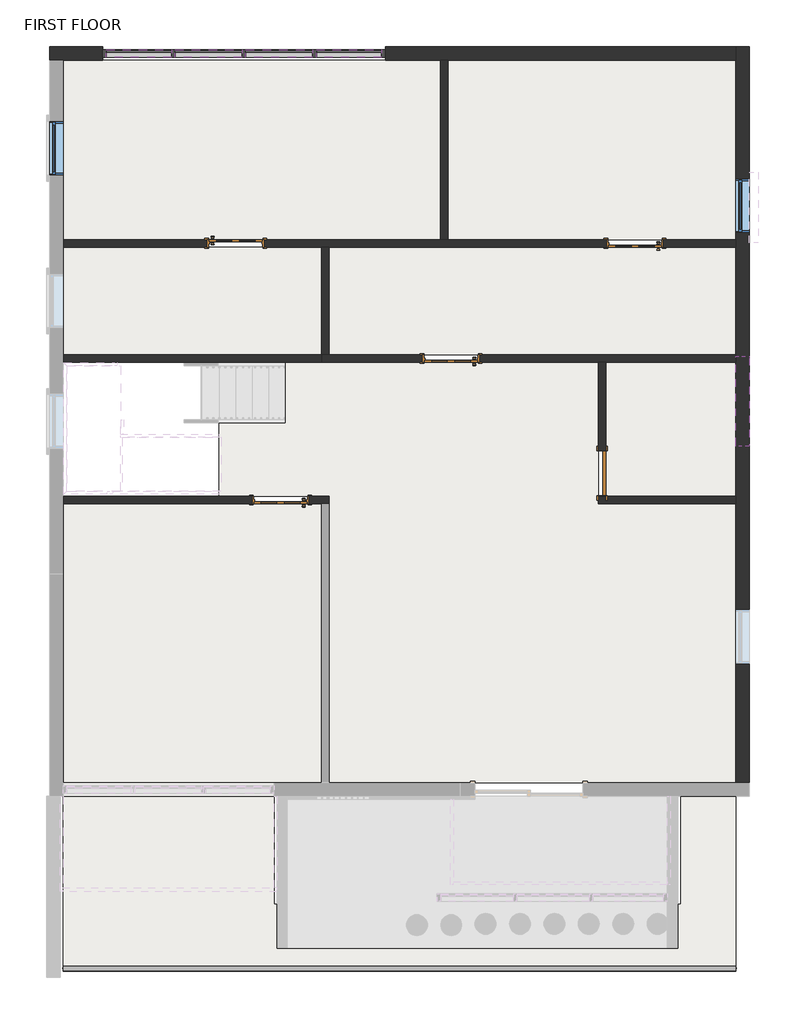
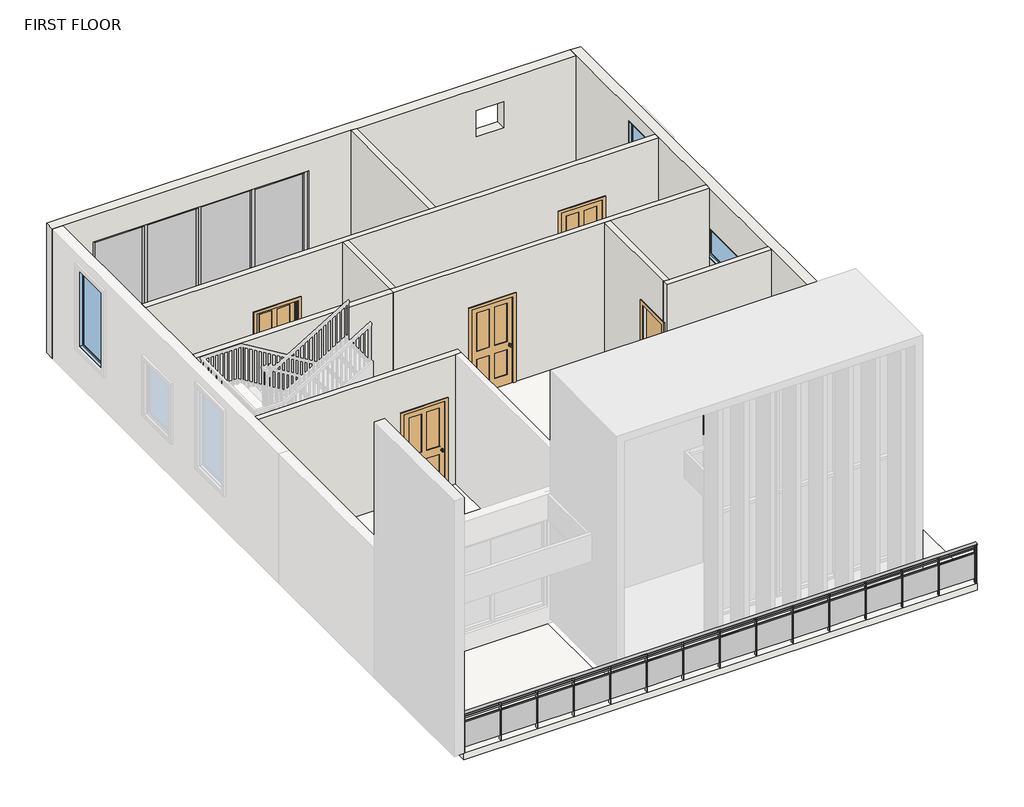
# One storey, part 2 of 4: 13 members, 10 walls, 5 doors, 4 plates, 3 windows, 1 railing, 1 slab.
"""IFC4 building model written with IfcOpenShell, lengths in millimetres."""

from ifc_helpers import new_model, si_unit, point, frame, origin, place, context, project, spatial, polyline, ellipse_curve, trimmed, outline, extrude, faceted_brep, transform, mapped, element, save
from ifc_brep_helpers import plane_surface, extruded_surface, advanced_brep
from components import door_65ef8926, door_1fe7f57d, member_d69c7880, member_a8685e1c, member_189d47d0, member_5afaafd3, system_panel_glazed_d43da186, system_panel_glazed_a1d10a75, window_2e8ca8a3, window_e88f44c6

model = new_model("IFC4")

# Units and contexts
model_context = context("Model", 3, world=origin())
ifc_project = project(units=[si_unit("LENGTHUNIT", "METRE", prefix="MILLI")], contexts=[model_context])

# Site, building, storey
site = spatial("IfcSite", under=ifc_project)
building = spatial("IfcBuilding", under=site)
storey = spatial("IfcBuildingStorey", under=building, Name="FIRST FLOOR", Elevation=3352.8)

# Doors
placement = place(None, origin())
door_shape = door_65ef8926(model_context)
element("IfcDoor", 1, ObjectType="Door-Interior-Single-4_Panel-Wood : 36\" x 80\"", at=placement, inside=storey, context=model_context, shape_type="MappedRepresentation", body=[
    mapped(door_shape, transform((-6068.2781265, 636.4415128, 3352.8), x_axis=(-1.0, 0.0, 0.0), y_axis=(0.0, -1.0, 0.0), z_axis=(0.0, 0.0, 1.0))),
])
element("IfcDoor", 2, ObjectType="Door-Interior-Single-4_Panel-Wood : 36\" x 80\"", at=placement, inside=storey, context=model_context, shape_type="MappedRepresentation", body=[
    mapped(door_shape, transform((-3172.6781265, 3037.1107468, 3352.8), x_axis=(-1.0, 0.0, 0.0), y_axis=(0.0, -1.0, 0.0), z_axis=(0.0, 0.0, 1.0))),
])
element("IfcDoor", 3, ObjectType="Door-Interior-Single-4_Panel-Wood : 36\" x 80\"", at=placement, inside=storey, context=model_context, shape_type="MappedRepresentation", body=[
    mapped(door_shape, transform((-6830.2781265, 4999.2607468, 3352.8), x_axis=(1.0, 0.0, 0.0), y_axis=(0.0, 1.0, 0.0), z_axis=(0.0, 0.0, 1.0))),
])
element("IfcDoor", 4, ObjectType="Door-Interior-Single-4_Panel-Wood : 36\" x 80\"", at=placement, inside=storey, context=model_context, shape_type="MappedRepresentation", body=[
    mapped(door_shape, transform((-48.4781265, 4992.9107468, 3352.8), x_axis=(-1.0, 0.0, 0.0), y_axis=(0.0, -1.0, 0.0), z_axis=(0.0, 0.0, 1.0))),
])
door_2_shape = door_1fe7f57d(model_context)
element("IfcDoor", 5, ObjectType="Single-Flush : 30\" x 80\"", at=placement, inside=storey, context=model_context, shape_type="MappedRepresentation", body=[
    mapped(door_2_shape, transform((-607.2781265, 1096.8165128, 3352.8), x_axis=(0.0, -1.0, 0.0), y_axis=(1.0, 0.0, 0.0), z_axis=(0.0, 0.0, 1.0))),
])

# Members
member_shape = member_d69c7880(model_context)
element("IfcMember", 6, ObjectType="Rectangular Mullion : 2.5\" x 5\" rectangular", at=placement, inside=storey, context=model_context, shape_type="MappedRepresentation", body=[
    mapped(member_shape, transform((-4353.7781265, 8221.8857468, 5781.7640157), x_axis=(0.0, 0.0, 1.0), y_axis=(0.0, -1.0, 0.0), z_axis=(1.0, 0.0, 0.0))),
])
element("IfcMember", 7, ObjectType="Rectangular Mullion : 2.5\" x 5\" rectangular", at=placement, inside=storey, context=model_context, shape_type="MappedRepresentation", body=[
    mapped(member_shape, transform((-7922.4781263, 8221.8857468, 5781.7640157), x_axis=(0.0, 0.0, 1.0), y_axis=(0.0, -1.0, 0.0), z_axis=(1.0, 0.0, 0.0))),
])
member_2_shape = member_a8685e1c(model_context)
element("IfcMember", 8, ObjectType="Rectangular Mullion : 2.5\" x 5\" rectangular", at=placement, inside=storey, context=model_context, shape_type="MappedRepresentation", body=[
    mapped(member_2_shape, transform((-6722.3281265, 8221.8857468, 5781.7640157), x_axis=(0.0, 0.0, 1.0), y_axis=(0.0, -1.0, 0.0), z_axis=(1.0, 0.0, 0.0))),
])
element("IfcMember", 9, ObjectType="Rectangular Mullion : 2.5\" x 5\" rectangular", at=placement, inside=storey, context=model_context, shape_type="MappedRepresentation", body=[
    mapped(member_2_shape, transform((-5522.1781266, 8221.8857468, 5781.7640157), x_axis=(0.0, 0.0, 1.0), y_axis=(0.0, -1.0, 0.0), z_axis=(1.0, 0.0, 0.0))),
])
element("IfcMember", 10, ObjectType="Rectangular Mullion : 2.5\" x 5\" rectangular", at=placement, inside=storey, context=model_context, shape_type="MappedRepresentation", body=[
    mapped(member_shape, transform((-9027.3781265, 8221.8857468, 3352.8), x_axis=(0.0, 0.0, -1.0), y_axis=(0.0, -1.0, 0.0), z_axis=(-1.0, 0.0, 0.0))),
])
element("IfcMember", 11, ObjectType="Rectangular Mullion : 2.5\" x 5\" rectangular", at=placement, inside=storey, context=model_context, shape_type="MappedRepresentation", body=[
    mapped(member_shape, transform((-5458.6781266, 8221.8857468, 3352.8), x_axis=(0.0, 0.0, -1.0), y_axis=(0.0, -1.0, 0.0), z_axis=(-1.0, 0.0, 0.0))),
])
element("IfcMember", 12, ObjectType="Rectangular Mullion : 2.5\" x 5\" rectangular", at=placement, inside=storey, context=model_context, shape_type="MappedRepresentation", body=[
    mapped(member_2_shape, transform((-7858.9781263, 8221.8857468, 3352.8), x_axis=(0.0, 0.0, -1.0), y_axis=(0.0, -1.0, 0.0), z_axis=(-1.0, 0.0, 0.0))),
])
element("IfcMember", 13, ObjectType="Rectangular Mullion : 2.5\" x 5\" rectangular", at=placement, inside=storey, context=model_context, shape_type="MappedRepresentation", body=[
    mapped(member_2_shape, transform((-6658.8281265, 8221.8857468, 3352.8), x_axis=(0.0, 0.0, -1.0), y_axis=(0.0, -1.0, 0.0), z_axis=(-1.0, 0.0, 0.0))),
])
member_3_shape = member_189d47d0(model_context)
element("IfcMember", 14, ObjectType="Rectangular Mullion : 2.5\" x 5\" rectangular", at=placement, inside=storey, context=model_context, shape_type="MappedRepresentation", body=[
    mapped(member_3_shape, transform((-7890.7281263, 8221.8857468, 3352.8), x_axis=(1.0, 0.0, 0.0), y_axis=(0.0, -1.0, 0.0), z_axis=(0.0, 0.0, -1.0))),
])
element("IfcMember", 15, ObjectType="Rectangular Mullion : 2.5\" x 5\" rectangular", at=placement, inside=storey, context=model_context, shape_type="MappedRepresentation", body=[
    mapped(member_3_shape, transform((-6690.5781265, 8221.8857468, 3352.8), x_axis=(1.0, 0.0, 0.0), y_axis=(0.0, -1.0, 0.0), z_axis=(0.0, 0.0, -1.0))),
])
element("IfcMember", 16, ObjectType="Rectangular Mullion : 2.5\" x 5\" rectangular", at=placement, inside=storey, context=model_context, shape_type="MappedRepresentation", body=[
    mapped(member_3_shape, transform((-5490.4281266, 8221.8857468, 3352.8), x_axis=(1.0, 0.0, 0.0), y_axis=(0.0, -1.0, 0.0), z_axis=(0.0, 0.0, -1.0))),
])
member_4_shape = member_5afaafd3(model_context)
element("IfcMember", 17, ObjectType="Rectangular Mullion : 2.5\" x 5\" rectangular", at=placement, inside=storey, context=model_context, shape_type="MappedRepresentation", body=[
    mapped(member_4_shape, transform((-4290.2781265, 8221.8857468, 3352.8), x_axis=(1.0, 0.0, 0.0), y_axis=(0.0, -1.0, 0.0), z_axis=(0.0, 0.0, -1.0))),
])
element("IfcMember", 18, ObjectType="Rectangular Mullion : 2.5\" x 5\" rectangular", at=placement, inside=storey, context=model_context, shape_type="MappedRepresentation", body=[
    mapped(member_4_shape, transform((-9090.8781265, 8221.8857468, 5781.7640157), x_axis=(-1.0, 0.0, 0.0), y_axis=(0.0, -1.0, 0.0), z_axis=(0.0, 0.0, 1.0))),
])

# Plates
system_panel_glazed_shape = system_panel_glazed_d43da186(model_context)
element("IfcPlate", 19, ObjectType="System Panel : Glazed", at=placement, inside=storey, context=model_context, shape_type="MappedRepresentation", body=[
    mapped(system_panel_glazed_shape, transform((-8474.9281264, 8221.8857468, 3416.3), x_axis=(1.0, 0.0, 0.0), y_axis=(0.0, 1.0, 0.0), z_axis=(0.0, 0.0, 1.0))),
])
element("IfcPlate", 20, ObjectType="System Panel : Glazed", at=placement, inside=storey, context=model_context, shape_type="MappedRepresentation", body=[
    mapped(system_panel_glazed_shape, transform((-4906.2281265, 8221.8857468, 3416.3), x_axis=(1.0, 0.0, 0.0), y_axis=(0.0, 1.0, 0.0), z_axis=(0.0, 0.0, 1.0))),
])
system_panel_glazed_2_shape = system_panel_glazed_a1d10a75(model_context)
element("IfcPlate", 21, ObjectType="System Panel : Glazed", at=placement, inside=storey, context=model_context, shape_type="MappedRepresentation", body=[
    mapped(system_panel_glazed_2_shape, transform((-7290.6531264, 8221.8857468, 3416.3), x_axis=(1.0, 0.0, 0.0), y_axis=(0.0, 1.0, 0.0), z_axis=(0.0, 0.0, 1.0))),
])
element("IfcPlate", 22, ObjectType="System Panel : Glazed", at=placement, inside=storey, context=model_context, shape_type="MappedRepresentation", body=[
    mapped(system_panel_glazed_2_shape, transform((-6090.5031265, 8221.8857468, 3416.3), x_axis=(1.0, 0.0, 0.0), y_axis=(0.0, 1.0, 0.0), z_axis=(0.0, 0.0, 1.0))),
])

# Railing
element("IfcRailing", 23, ObjectType="Glass Panel - Bottom Fill", at=placement, inside=storey, context=model_context, shape_type="SolidModel", body=[
    advanced_brep(
    [(-9763.9781265, -7272.1142532, 4267.2), (-9763.9781265, -7348.3142532, 4267.2), (1666.0218735, -7272.1142532, 4267.2), (1666.0218735, -7348.3142532, 4267.2)],
    [
        (0, 1, ellipse_curve(frame((-9763.9781265, -7310.2142532, 4267.2), z_axis=(-1.0, 0.0, 0.0), x_axis=(0.0, -1.0, 0.0)), 38.1, 28.575)),
        (1, 0, ellipse_curve(frame((-9763.9781265, -7310.2142532, 4267.2), z_axis=(-1.0, 0.0, 0.0), x_axis=(0.0, -1.0, 0.0)), 38.1, 28.575)),
        (2, 3, ellipse_curve(frame((1666.0218735, -7310.2142532, 4267.2), z_axis=(1.0, 0.0, 0.0), x_axis=(0.0, -1.0, 0.0)), 38.1, 28.575)),
        (3, 2, ellipse_curve(frame((1666.0218735, -7310.2142532, 4267.2), z_axis=(1.0, 0.0, 0.0), x_axis=(0.0, -1.0, 0.0)), 38.1, 28.575)),
        (0, 2),
        (3, 1),
    ],
    [
        plane_surface(frame((-9763.9781265, -7310.2142532, 4267.2), z_axis=(-1.0, 0.0, 0.0), x_axis=(0.0, 1.0, 0.0))),
        plane_surface(frame((1666.0218735, -7310.2142532, 4267.2), z_axis=(1.0, 0.0, 0.0), x_axis=(0.0, 1.0, 0.0))),
        extruded_surface(trimmed(ellipse_curve(frame((1666.0218735, -7310.2142532, 4267.2), z_axis=(-1.0, 0.0, 0.0), x_axis=(0.0, -1.0, 0.0)), 38.1, 28.575), [point((1666.0218735, -7272.1142532, 4267.2))], [point((1666.0218735, -7348.3142532, 4267.2))], True, "CARTESIAN"), (-11430.0, 0.0, 0.0), 11430.0),
        extruded_surface(trimmed(ellipse_curve(frame((1666.0218735, -7310.2142532, 4267.2), z_axis=(-1.0, 0.0, 0.0), x_axis=(0.0, -1.0, 0.0)), 38.1, 28.575), [point((1666.0218735, -7348.3142532, 4267.2))], [point((1666.0218735, -7272.1142532, 4267.2))], True, "CARTESIAN"), (-11430.0, 0.0, 0.0), 11430.0),
    ],
    [
        (0, [[1, 2]]),
        (1, [[3, 4]]),
        (2, [[-1, 5, -4, 6]]),
        (3, [[-2, -6, -3, -5]]),
    ],
),
    extrude(outline(polyline([(-9763.9781265, -7322.9142532), (-9763.9781265, -7297.5142532), (1666.0218735, -7297.5142532), (1666.0218735, -7322.9142532), (-9763.9781265, -7322.9142532)])), frame((0.0, 0.0, 4152.9), z_axis=(0.0, 0.0, 1.0), x_axis=(1.0, 0.0, 0.0)), (0.0, 0.0, 1.0), 25.4),
    extrude(outline(polyline([(-9763.9781265, -7322.9142532), (-9763.9781265, -7297.5142532), (1666.0218735, -7297.5142532), (1666.0218735, -7322.9142532), (-9763.9781265, -7322.9142532)])), frame((0.0, 0.0, 4051.3), z_axis=(0.0, 0.0, 1.0), x_axis=(1.0, 0.0, 0.0)), (0.0, 0.0, 1.0), 25.4),
    extrude(outline(polyline([(1634.2718735, -7335.6142532), (1634.2718735, -7284.8142532), (1646.9718735, -7284.8142532), (1646.9718735, -7335.6142532), (1634.2718735, -7335.6142532)])), frame((0.0, 0.0, 3352.8), z_axis=(0.0, 0.0, 1.0), x_axis=(1.0, 0.0, 0.0)), (0.0, 0.0, 1.0), 885.825),
    extrude(outline(polyline([(827.8218735, -7303.6790962), (1640.6218735, -7303.6790962), (1640.6218735, -7310.0290962), (827.8218735, -7310.0290962), (827.8218735, -7303.6790962)])), frame((0.0, 0.0, 3454.4), z_axis=(0.0, 0.0, 1.0), x_axis=(1.0, 0.0, 0.0)), (0.0, 0.0, 1.0), 596.9),
    extrude(outline(polyline([(821.4718735, -7335.6142532), (821.4718735, -7284.8142532), (834.1718735, -7284.8142532), (834.1718735, -7335.6142532), (821.4718735, -7335.6142532)])), frame((0.0, 0.0, 3352.8), z_axis=(0.0, 0.0, 1.0), x_axis=(1.0, 0.0, 0.0)), (0.0, 0.0, 1.0), 885.825),
    extrude(outline(polyline([(15.0218735, -7303.6790962), (827.8218735, -7303.6790962), (827.8218735, -7310.0290962), (15.0218735, -7310.0290962), (15.0218735, -7303.6790962)])), frame((0.0, 0.0, 3454.4), z_axis=(0.0, 0.0, 1.0), x_axis=(1.0, 0.0, 0.0)), (0.0, 0.0, 1.0), 596.9),
    extrude(outline(polyline([(8.6718735, -7335.6142532), (8.6718735, -7284.8142532), (21.3718735, -7284.8142532), (21.3718735, -7335.6142532), (8.6718735, -7335.6142532)])), frame((0.0, 0.0, 3352.8), z_axis=(0.0, 0.0, 1.0), x_axis=(1.0, 0.0, 0.0)), (0.0, 0.0, 1.0), 885.825),
    extrude(outline(polyline([(-797.7781265, -7303.6790962), (15.0218735, -7303.6790962), (15.0218735, -7310.0290962), (-797.7781265, -7310.0290962), (-797.7781265, -7303.6790962)])), frame((0.0, 0.0, 3454.4), z_axis=(0.0, 0.0, 1.0), x_axis=(1.0, 0.0, 0.0)), (0.0, 0.0, 1.0), 596.9),
    extrude(outline(polyline([(-804.1281265, -7335.6142532), (-804.1281265, -7284.8142532), (-791.4281265, -7284.8142532), (-791.4281265, -7335.6142532), (-804.1281265, -7335.6142532)])), frame((0.0, 0.0, 3352.8), z_axis=(0.0, 0.0, 1.0), x_axis=(1.0, 0.0, 0.0)), (0.0, 0.0, 1.0), 885.825),
    extrude(outline(polyline([(-1610.5781265, -7303.6790962), (-797.7781265, -7303.6790962), (-797.7781265, -7310.0290962), (-1610.5781265, -7310.0290962), (-1610.5781265, -7303.6790962)])), frame((0.0, 0.0, 3454.4), z_axis=(0.0, 0.0, 1.0), x_axis=(1.0, 0.0, 0.0)), (0.0, 0.0, 1.0), 596.9),
    extrude(outline(polyline([(-1616.9281265, -7335.6142532), (-1616.9281265, -7284.8142532), (-1604.2281265, -7284.8142532), (-1604.2281265, -7335.6142532), (-1616.9281265, -7335.6142532)])), frame((0.0, 0.0, 3352.8), z_axis=(0.0, 0.0, 1.0), x_axis=(1.0, 0.0, 0.0)), (0.0, 0.0, 1.0), 885.825),
    extrude(outline(polyline([(-2423.3781265, -7303.6790962), (-1610.5781265, -7303.6790962), (-1610.5781265, -7310.0290962), (-2423.3781265, -7310.0290962), (-2423.3781265, -7303.6790962)])), frame((0.0, 0.0, 3454.4), z_axis=(0.0, 0.0, 1.0), x_axis=(1.0, 0.0, 0.0)), (0.0, 0.0, 1.0), 596.9),
    extrude(outline(polyline([(-2429.7281265, -7335.6142532), (-2429.7281265, -7284.8142532), (-2417.0281265, -7284.8142532), (-2417.0281265, -7335.6142532), (-2429.7281265, -7335.6142532)])), frame((0.0, 0.0, 3352.8), z_axis=(0.0, 0.0, 1.0), x_axis=(1.0, 0.0, 0.0)), (0.0, 0.0, 1.0), 885.825),
    extrude(outline(polyline([(-3236.1781265, -7303.6790962), (-2423.3781265, -7303.6790962), (-2423.3781265, -7310.0290962), (-3236.1781265, -7310.0290962), (-3236.1781265, -7303.6790962)])), frame((0.0, 0.0, 3454.4), z_axis=(0.0, 0.0, 1.0), x_axis=(1.0, 0.0, 0.0)), (0.0, 0.0, 1.0), 596.9),
    extrude(outline(polyline([(-3242.5281265, -7335.6142532), (-3242.5281265, -7284.8142532), (-3229.8281265, -7284.8142532), (-3229.8281265, -7335.6142532), (-3242.5281265, -7335.6142532)])), frame((0.0, 0.0, 3352.8), z_axis=(0.0, 0.0, 1.0), x_axis=(1.0, 0.0, 0.0)), (0.0, 0.0, 1.0), 885.825),
    extrude(outline(polyline([(-4048.9781265, -7303.6790962), (-3236.1781265, -7303.6790962), (-3236.1781265, -7310.0290962), (-4048.9781265, -7310.0290962), (-4048.9781265, -7303.6790962)])), frame((0.0, 0.0, 3454.4), z_axis=(0.0, 0.0, 1.0), x_axis=(1.0, 0.0, 0.0)), (0.0, 0.0, 1.0), 596.9),
    extrude(outline(polyline([(-4055.3281265, -7335.6142532), (-4055.3281265, -7284.8142532), (-4042.6281265, -7284.8142532), (-4042.6281265, -7335.6142532), (-4055.3281265, -7335.6142532)])), frame((0.0, 0.0, 3352.8), z_axis=(0.0, 0.0, 1.0), x_axis=(1.0, 0.0, 0.0)), (0.0, 0.0, 1.0), 885.825),
    extrude(outline(polyline([(-4861.7781265, -7303.6790962), (-4048.9781265, -7303.6790962), (-4048.9781265, -7310.0290962), (-4861.7781265, -7310.0290962), (-4861.7781265, -7303.6790962)])), frame((0.0, 0.0, 3454.4), z_axis=(0.0, 0.0, 1.0), x_axis=(1.0, 0.0, 0.0)), (0.0, 0.0, 1.0), 596.9),
    extrude(outline(polyline([(-4868.1281265, -7335.6142532), (-4868.1281265, -7284.8142532), (-4855.4281265, -7284.8142532), (-4855.4281265, -7335.6142532), (-4868.1281265, -7335.6142532)])), frame((0.0, 0.0, 3352.8), z_axis=(0.0, 0.0, 1.0), x_axis=(1.0, 0.0, 0.0)), (0.0, 0.0, 1.0), 885.825),
    extrude(outline(polyline([(-5674.5781265, -7303.6790962), (-4861.7781265, -7303.6790962), (-4861.7781265, -7310.0290962), (-5674.5781265, -7310.0290962), (-5674.5781265, -7303.6790962)])), frame((0.0, 0.0, 3454.4), z_axis=(0.0, 0.0, 1.0), x_axis=(1.0, 0.0, 0.0)), (0.0, 0.0, 1.0), 596.9),
    extrude(outline(polyline([(-5680.9281265, -7335.6142532), (-5680.9281265, -7284.8142532), (-5668.2281265, -7284.8142532), (-5668.2281265, -7335.6142532), (-5680.9281265, -7335.6142532)])), frame((0.0, 0.0, 3352.8), z_axis=(0.0, 0.0, 1.0), x_axis=(1.0, 0.0, 0.0)), (0.0, 0.0, 1.0), 885.825),
    extrude(outline(polyline([(-6487.3781265, -7303.6790962), (-5674.5781265, -7303.6790962), (-5674.5781265, -7310.0290962), (-6487.3781265, -7310.0290962), (-6487.3781265, -7303.6790962)])), frame((0.0, 0.0, 3454.4), z_axis=(0.0, 0.0, 1.0), x_axis=(1.0, 0.0, 0.0)), (0.0, 0.0, 1.0), 596.9),
    extrude(outline(polyline([(-6493.7281265, -7335.6142532), (-6493.7281265, -7284.8142532), (-6481.0281265, -7284.8142532), (-6481.0281265, -7335.6142532), (-6493.7281265, -7335.6142532)])), frame((0.0, 0.0, 3352.8), z_axis=(0.0, 0.0, 1.0), x_axis=(1.0, 0.0, 0.0)), (0.0, 0.0, 1.0), 885.825),
    extrude(outline(polyline([(-7300.1781265, -7303.6790962), (-6487.3781265, -7303.6790962), (-6487.3781265, -7310.0290962), (-7300.1781265, -7310.0290962), (-7300.1781265, -7303.6790962)])), frame((0.0, 0.0, 3454.4), z_axis=(0.0, 0.0, 1.0), x_axis=(1.0, 0.0, 0.0)), (0.0, 0.0, 1.0), 596.9),
    extrude(outline(polyline([(-7306.5281265, -7335.6142532), (-7306.5281265, -7284.8142532), (-7293.8281265, -7284.8142532), (-7293.8281265, -7335.6142532), (-7306.5281265, -7335.6142532)])), frame((0.0, 0.0, 3352.8), z_axis=(0.0, 0.0, 1.0), x_axis=(1.0, 0.0, 0.0)), (0.0, 0.0, 1.0), 885.825),
    extrude(outline(polyline([(-8112.9781265, -7303.6790962), (-7300.1781265, -7303.6790962), (-7300.1781265, -7310.0290962), (-8112.9781265, -7310.0290962), (-8112.9781265, -7303.6790962)])), frame((0.0, 0.0, 3454.4), z_axis=(0.0, 0.0, 1.0), x_axis=(1.0, 0.0, 0.0)), (0.0, 0.0, 1.0), 596.9),
    extrude(outline(polyline([(-8119.3281265, -7335.6142532), (-8119.3281265, -7284.8142532), (-8106.6281265, -7284.8142532), (-8106.6281265, -7335.6142532), (-8119.3281265, -7335.6142532)])), frame((0.0, 0.0, 3352.8), z_axis=(0.0, 0.0, 1.0), x_axis=(1.0, 0.0, 0.0)), (0.0, 0.0, 1.0), 885.825),
    extrude(outline(polyline([(-8925.7781265, -7303.6790962), (-8112.9781265, -7303.6790962), (-8112.9781265, -7310.0290962), (-8925.7781265, -7310.0290962), (-8925.7781265, -7303.6790962)])), frame((0.0, 0.0, 3454.4), z_axis=(0.0, 0.0, 1.0), x_axis=(1.0, 0.0, 0.0)), (0.0, 0.0, 1.0), 596.9),
    extrude(outline(polyline([(-8932.1281265, -7335.6142532), (-8932.1281265, -7284.8142532), (-8919.4281265, -7284.8142532), (-8919.4281265, -7335.6142532), (-8932.1281265, -7335.6142532)])), frame((0.0, 0.0, 3352.8), z_axis=(0.0, 0.0, 1.0), x_axis=(1.0, 0.0, 0.0)), (0.0, 0.0, 1.0), 885.825),
    extrude(outline(polyline([(-9738.5781265, -7303.6790962), (-8925.7781265, -7303.6790962), (-8925.7781265, -7310.0290962), (-9738.5781265, -7310.0290962), (-9738.5781265, -7303.6790962)])), frame((0.0, 0.0, 3454.4), z_axis=(0.0, 0.0, 1.0), x_axis=(1.0, 0.0, 0.0)), (0.0, 0.0, 1.0), 596.9),
    extrude(outline(polyline([(-9744.9281265, -7335.6142532), (-9744.9281265, -7284.8142532), (-9732.2281265, -7284.8142532), (-9732.2281265, -7335.6142532), (-9744.9281265, -7335.6142532)])), frame((0.0, 0.0, 3352.8), z_axis=(0.0, 0.0, 1.0), x_axis=(1.0, 0.0, 0.0)), (0.0, 0.0, 1.0), 885.825),
    extrude(outline(polyline([(1653.3218735, -7319.7392532), (1653.3218735, -7300.6892532), (1672.3718735, -7300.6892532), (1672.3718735, -7319.7392532), (1653.3218735, -7319.7392532)])), frame((0.0, 0.0, 3352.8), z_axis=(0.0, 0.0, 1.0), x_axis=(1.0, 0.0, 0.0)), (0.0, 0.0, 1.0), 885.825),
    extrude(outline(polyline([(-9770.3281265, -7319.7392532), (-9770.3281265, -7300.6892532), (-9751.2781265, -7300.6892532), (-9751.2781265, -7319.7392532), (-9770.3281265, -7319.7392532)])), frame((0.0, 0.0, 3352.8), z_axis=(0.0, 0.0, 1.0), x_axis=(1.0, 0.0, 0.0)), (0.0, 0.0, 1.0), 885.825),
])

# Slab
element("IfcSlab", 24, ObjectType="MARBLE FLOORING 6\"", at=placement, inside=storey, context=model_context, shape_type="SweptSolid", body=[
    extrude(outline(polyline([(-3350.4781265, 8107.5857468), (-3350.4781265, 5059.5857468), (-9763.9781265, 5059.5857468), (-9763.9781265, 8107.5857468), (-3350.4781265, 8107.5857468)])), frame((0.0, 0.0, 3200.4), z_axis=(0.0, 0.0, 1.0), x_axis=(1.0, 0.0, 0.0)), (0.0, 0.0, 1.0), 152.4),
    extrude(outline(polyline([(1666.0218735, 8107.5857468), (1666.0218735, 5059.5857468), (-3223.4781265, 5059.5857468), (-3223.4781265, 8107.5857468), (1666.0218735, 8107.5857468)])), frame((0.0, 0.0, 3200.4), z_axis=(0.0, 0.0, 1.0), x_axis=(1.0, 0.0, 0.0)), (0.0, 0.0, 1.0), 152.4),
    extrude(outline(polyline([(-5369.7781265, 4932.5857468), (-5369.7781265, 3103.7857468), (-9763.9781265, 3103.7857468), (-9763.9781265, 4932.5857468), (-5369.7781265, 4932.5857468)])), frame((0.0, 0.0, 3200.4), z_axis=(0.0, 0.0, 1.0), x_axis=(1.0, 0.0, 0.0)), (0.0, 0.0, 1.0), 152.4),
    extrude(outline(polyline([(1666.0218735, 4932.5857468), (1666.0218735, 3103.7857468), (-5242.7781265, 3103.7857468), (-5242.7781265, 4932.5857468), (1666.0218735, 4932.5857468)])), frame((0.0, 0.0, 3200.4), z_axis=(0.0, 0.0, 1.0), x_axis=(1.0, 0.0, 0.0)), (0.0, 0.0, 1.0), 152.4),
    extrude(outline(polyline([(1666.0218735, 703.1165128), (-543.7781265, 703.1165128), (-543.7781265, 2976.7857468), (1666.0218735, 2976.7857468), (1666.0218735, 703.1165128)])), frame((0.0, 0.0, 3200.4), z_axis=(0.0, 0.0, 1.0), x_axis=(1.0, 0.0, 0.0)), (0.0, 0.0, 1.0), 152.4),
    extrude(outline(polyline([(-5369.7781265, -4160.6142532), (-9763.9781265, -4160.6142532), (-9763.9781265, 576.1165128), (-5369.7781265, 576.1165128), (-5369.7781265, -4160.6142532)])), frame((0.0, 0.0, 3200.4), z_axis=(0.0, 0.0, 1.0), x_axis=(1.0, 0.0, 0.0)), (0.0, 0.0, 1.0), 152.4),
    extrude(outline(polyline([(497.6218735, -5989.4142532), (-5953.9781265, -5989.4142532), (-5953.9781265, -4389.2142532), (497.6218735, -4389.2142532), (497.6218735, -5989.4142532)])), frame((0.0, 0.0, 3200.4), z_axis=(0.0, 0.0, 1.0), x_axis=(1.0, 0.0, 0.0)), (0.0, 0.0, 1.0), 152.4),
    extrude(outline(polyline([(-6182.5781265, -4389.2142532), (-6182.5781265, -6218.0142532), (726.2218735, -6218.0142532), (726.2218735, -4389.2142532), (1666.0218735, -4389.2142532), (1666.0218735, -7361.0142532), (-9763.9781265, -7361.0142532), (-9763.9781265, -4389.2142532), (-6182.5781265, -4389.2142532)])), frame((0.0, 0.0, 3200.4), z_axis=(0.0, 0.0, 1.0), x_axis=(1.0, 0.0, 0.0)), (0.0, 0.0, 1.0), 152.4),
    extrude(outline(polyline([(-5242.7781265, -4160.6142532), (-5242.7781265, 703.1165128), (-7108.4517085, 703.1165128), (-7108.4517085, 1953.8826226), (-5990.8517085, 1953.8826226), (-5990.8517085, 2976.7857468), (-670.7781265, 2976.7857468), (-670.7781265, 576.1165128), (1666.0218735, 576.1165128), (1666.0218735, -4160.6142532), (-5242.7781265, -4160.6142532)])), frame((0.0, 0.0, 3200.4), z_axis=(0.0, 0.0, 1.0), x_axis=(1.0, 0.0, 0.0)), (0.0, 0.0, 1.0), 152.4),
])

# Walls
element("IfcWall", 25, ObjectType="Generic - 5\"", at=placement, inside=storey, context=model_context, shape_type="Brep", body=[
    faceted_brep([(1666.0218735, 4932.5857468, 6400.8), (-5242.7781265, 4932.5857468, 6400.8), (-5369.7781265, 4932.5857468, 6400.8), (-9763.9781265, 4932.5857468, 6400.8), (-9763.9781265, 4932.5857468, 3352.8), (-7312.8781265, 4932.5857468, 3352.8), (-7312.8781265, 4932.5857468, 5410.2), (-6347.6781265, 4932.5857468, 5410.2), (-6347.6781265, 4932.5857468, 3352.8), (-5369.7781265, 4932.5857468, 3352.8), (-5242.7781265, 4932.5857468, 3352.8), (-531.0781265, 4932.5857468, 3352.8), (-531.0781265, 4932.5857468, 5410.2), (434.1218735, 4932.5857468, 5410.2), (434.1218735, 4932.5857468, 3352.8), (1666.0218735, 4932.5857468, 3352.8), (-9763.9781265, 5059.5857468, 6400.8), (-3350.4781265, 5059.5857468, 6400.8), (-3223.4781265, 5059.5857468, 6400.8), (1666.0218735, 5059.5857468, 6400.8), (1666.0218735, 5059.5857468, 3352.8), (434.1218735, 5059.5857468, 3352.8), (434.1218735, 5059.5857468, 5410.2), (-531.0781265, 5059.5857468, 5410.2), (-531.0781265, 5059.5857468, 3352.8), (-3223.4781265, 5059.5857468, 3352.8), (-3350.4781265, 5059.5857468, 3352.8), (-6347.6781265, 5059.5857468, 3352.8), (-6347.6781265, 5059.5857468, 5410.2), (-7312.8781265, 5059.5857468, 5410.2), (-7312.8781265, 5059.5857468, 3352.8), (-9763.9781265, 5059.5857468, 3352.8)], [[[0, 1, 2, 3, 4, 5, 6, 7, 8, 9, 10, 11, 12, 13, 14, 15]], [[16, 17, 18, 19, 20, 21, 22, 23, 24, 25, 26, 27, 28, 29, 30, 31]], [[4, 31, 30, 5]], [[20, 15, 14, 21]], [[8, 27, 26, 25, 24, 11, 10, 9]], [[3, 2, 1, 0, 19, 18, 17, 16]], [[4, 3, 16, 31]], [[0, 15, 20, 19]], [[7, 28, 27, 8]], [[28, 7, 6, 29]], [[29, 6, 5, 30]], [[23, 12, 11, 24]], [[12, 23, 22, 13]], [[13, 22, 21, 14]]]),
])
element("IfcWall", 26, ObjectType="Generic - 5\"", at=placement, inside=storey, context=model_context, shape_type="SweptSolid", body=[
    extrude(outline(polyline([(-5369.7781265, 3103.7857468), (-5369.7781265, 4932.5857468), (-5242.7781265, 4932.5857468), (-5242.7781265, 3103.7857468), (-5369.7781265, 3103.7857468)])), frame((0.0, 0.0, 3352.8), z_axis=(0.0, 0.0, 1.0), x_axis=(1.0, 0.0, 0.0)), (0.0, 0.0, 1.0), 3048.0),
])
element("IfcWall", 27, ObjectType="Generic - 5\"", at=placement, inside=storey, context=model_context, shape_type="SweptSolid", body=[
    extrude(outline(polyline([(-9763.9781265, 3103.7857468), (-5369.7781265, 3103.7857468), (-5369.7781265, 2976.7857468), (-9763.9781265, 2976.7857468), (-9763.9781265, 3103.7857468)])), frame((0.0, 0.0, 3352.8), z_axis=(0.0, 0.0, 1.0), x_axis=(1.0, 0.0, 0.0)), (0.0, 0.0, 1.0), 3048.0),
])
element("IfcWall", 28, ObjectType="INNER WALL THICKNESS 5\"", at=placement, inside=storey, context=model_context, shape_type="Brep", body=[
    faceted_brep([(-5242.7781265, 576.1165128, 6400.8), (-5369.7781265, 576.1165128, 6400.8), (-9763.9781265, 576.1165128, 6400.8), (-9763.9781265, 576.1165128, 3352.8), (-6550.8781265, 576.1165128, 3352.8), (-6550.8781265, 576.1165128, 5410.2), (-5585.6781265, 576.1165128, 5410.2), (-5585.6781265, 576.1165128, 3352.8), (-5369.7781265, 576.1165128, 3352.8), (-5242.7781265, 576.1165128, 3352.8), (-9763.9781265, 703.1165128, 6400.8), (-5242.7781265, 703.1165128, 6400.8), (-5242.7781265, 703.1165128, 3352.8), (-5585.6781265, 703.1165128, 3352.8), (-5585.6781265, 703.1165128, 5410.2), (-6550.8781265, 703.1165128, 5410.2), (-6550.8781265, 703.1165128, 3352.8), (-9763.9781265, 703.1165128, 3352.8)], [[[0, 1, 2, 3, 4, 5, 6, 7, 8, 9]], [[10, 11, 12, 13, 14, 15, 16, 17]], [[3, 17, 16, 4]], [[12, 9, 8, 7, 13]], [[2, 1, 0, 11, 10]], [[3, 2, 10, 17]], [[0, 9, 12, 11]], [[15, 5, 4, 16]], [[5, 15, 14, 6]], [[6, 14, 13, 7]]]),
])
element("IfcWall", 29, ObjectType="INNER WALL THICKNESS 5\"", at=placement, inside=storey, context=model_context, shape_type="Brep", body=[
    faceted_brep([(1666.0218735, 703.1165128, 3352.8), (-543.7781265, 703.1165128, 3352.8), (-670.7781265, 703.1165128, 3352.8), (-670.7781265, 703.1165128, 6400.8), (-543.7781265, 703.1165128, 6400.8), (1666.0218735, 703.1165128, 6400.8), (1666.0218735, 576.1165128, 3352.8), (1666.0218735, 576.1165128, 6400.8), (-670.7781265, 576.1165128, 6400.8), (-670.7781265, 576.1165128, 3352.8)], [[[0, 1, 2, 3, 4, 5]], [[6, 7, 8, 9]], [[2, 1, 0, 6, 9]], [[5, 4, 3, 8, 7]], [[0, 5, 7, 6]], [[3, 2, 9, 8]]]),
])
element("IfcWall", 30, ObjectType="INNER WALL THICKNESS 5\"", at=placement, inside=storey, context=model_context, shape_type="SweptSolid", body=[
    extrude(outline(polyline([(715.8165128, 5384.8), (715.8165128, 3352.8), (703.1165128, 3352.8), (703.1165128, 6400.8), (2976.7857468, 6400.8), (2976.7857468, 3352.8), (1477.8165128, 3352.8), (1477.8165128, 5384.8), (715.8165128, 5384.8)])), frame((-670.7781265, 0.0, 0.0), z_axis=(1.0, 0.0, 0.0), x_axis=(0.0, 1.0, 0.0)), (0.0, 0.0, 1.0), 127.0),
])
element("IfcWall", 31, ObjectType="INNER WALL THICKNESS 5\"", at=placement, inside=storey, context=model_context, shape_type="Brep", body=[
    faceted_brep([(1666.0218735, 2976.7857468, 6400.8), (-543.7781265, 2976.7857468, 6400.8), (-670.7781265, 2976.7857468, 6400.8), (-5369.7781265, 2976.7857468, 6400.8), (-5369.7781265, 2976.7857468, 3352.8), (-3655.2781265, 2976.7857468, 3352.8), (-3655.2781265, 2976.7857468, 5410.2), (-2690.0781265, 2976.7857468, 5410.2), (-2690.0781265, 2976.7857468, 3352.8), (-670.7781265, 2976.7857468, 3352.8), (-543.7781265, 2976.7857468, 3352.8), (1666.0218735, 2976.7857468, 3352.8), (-5369.7781265, 3103.7857468, 6400.8), (-5242.7781265, 3103.7857468, 6400.8), (1666.0218735, 3103.7857468, 6400.8), (1666.0218735, 3103.7857468, 3352.8), (-2690.0781265, 3103.7857468, 3352.8), (-2690.0781265, 3103.7857468, 5410.2), (-3655.2781265, 3103.7857468, 5410.2), (-3655.2781265, 3103.7857468, 3352.8), (-5242.7781265, 3103.7857468, 3352.8), (-5369.7781265, 3103.7857468, 3352.8)], [[[0, 1, 2, 3, 4, 5, 6, 7, 8, 9, 10, 11]], [[12, 13, 14, 15, 16, 17, 18, 19, 20, 21]], [[15, 11, 10, 9, 8, 16]], [[4, 21, 20, 19, 5]], [[3, 2, 1, 0, 14, 13, 12]], [[0, 11, 15, 14]], [[4, 3, 12, 21]], [[18, 6, 5, 19]], [[6, 18, 17, 7]], [[7, 17, 16, 8]]]),
])
element("IfcWall", 32, ObjectType="INNER WALL THICKNESS 5\"", at=placement, inside=storey, context=model_context, shape_type="SweptSolid", body=[
    extrude(outline(polyline([(-3350.4781265, 5059.5857468), (-3350.4781265, 8107.5857468), (-3223.4781265, 8107.5857468), (-3223.4781265, 5059.5857468), (-3350.4781265, 5059.5857468)])), frame((0.0, 0.0, 3352.8), z_axis=(0.0, 0.0, 1.0), x_axis=(1.0, 0.0, 0.0)), (0.0, 0.0, 1.0), 3048.0),
])
element("IfcWall", 33, ObjectType="OUTER WALL THICKNESS 9\"", at=placement, inside=storey, context=model_context, shape_type="Brep", body=[
    faceted_brep([(1894.6218735, -4160.6142532, 3352.8), (1894.6218735, 8336.1857468, 3352.8), (1894.6218735, 8336.1857468, 6400.8), (1894.6218735, -4160.6142532, 6400.8), (1894.6218735, 6088.2857468, 6096.0), (1894.6218735, 6088.2857468, 4267.2), (1894.6218735, 5173.8857468, 4267.2), (1894.6218735, 5173.8857468, 6096.0), (1894.6218735, -1226.9142532, 6096.0), (1894.6218735, -1226.9142532, 4267.2), (1894.6218735, -2141.3142532, 4267.2), (1894.6218735, -2141.3142532, 6096.0), (1894.6218735, 3078.0165128, 5448.2767967), (1894.6218735, 3078.0165128, 4762.4767967), (1894.6218735, 1554.0165128, 4762.4767967), (1894.6218735, 1554.0165128, 5448.2767967), (1666.0218735, -4160.6142532, 3352.8), (1666.0218735, -4160.6142532, 6400.8), (1666.0218735, 576.1165128, 6400.8), (1666.0218735, 703.1165128, 6400.8), (1666.0218735, 2976.7857468, 6400.8), (1666.0218735, 3103.7857468, 6400.8), (1666.0218735, 4932.5857468, 6400.8), (1666.0218735, 5059.5857468, 6400.8), (1666.0218735, 8107.5857468, 6400.8), (1666.0218735, 8336.1857468, 6400.8), (1666.0218735, 8336.1857468, 3352.8), (1666.0218735, 8107.5857468, 3352.8), (1666.0218735, 5059.5857468, 3352.8), (1666.0218735, 4932.5857468, 3352.8), (1666.0218735, 3103.7857468, 3352.8), (1666.0218735, 2976.7857468, 3352.8), (1666.0218735, 703.1165128, 3352.8), (1666.0218735, 576.1165128, 3352.8), (1666.0218735, 6088.2857468, 6096.0), (1666.0218735, 5173.8857468, 6096.0), (1666.0218735, 5173.8857468, 4267.2), (1666.0218735, 6088.2857468, 4267.2), (1666.0218735, -1226.9142532, 6096.0), (1666.0218735, -2141.3142532, 6096.0), (1666.0218735, -2141.3142532, 4267.2), (1666.0218735, -1226.9142532, 4267.2), (1666.0218735, 3078.0165128, 5448.2767967), (1666.0218735, 1554.0165128, 5448.2767967), (1666.0218735, 1554.0165128, 4762.4767967), (1666.0218735, 3078.0165128, 4762.4767967)], [[[0, 1, 2, 3], [4, 5, 6, 7], [8, 9, 10, 11], [12, 13, 14, 15]], [[16, 17, 18, 19, 20, 21, 22, 23, 24, 25, 26, 27, 28, 29, 30, 31, 32, 33], [34, 35, 36, 37], [38, 39, 40, 41], [42, 43, 44, 45]], [[1, 0, 16, 33, 32, 31, 30, 29, 28, 27, 26]], [[3, 2, 25, 24, 23, 22, 21, 20, 19, 18, 17]], [[2, 1, 26, 25]], [[5, 4, 34, 37]], [[6, 5, 37, 36]], [[7, 6, 36, 35]], [[4, 7, 35, 34]], [[9, 8, 38, 41]], [[10, 9, 41, 40]], [[11, 10, 40, 39]], [[8, 11, 39, 38]], [[13, 12, 42, 45]], [[14, 13, 45, 44]], [[15, 14, 44, 43]], [[12, 15, 43, 42]], [[0, 3, 17, 16]]]),
])
element("IfcWall", 34, ObjectType="OUTER WALL THICKNESS 9\"", at=placement, inside=storey, context=model_context, shape_type="Brep", body=[
    faceted_brep([(-9992.5781265, 8336.1857468, 6400.8), (1666.0218735, 8336.1857468, 6400.8), (1666.0218735, 8336.1857468, 3352.8), (-4290.2781265, 8336.1857468, 3352.8), (-4290.2781265, 8336.1857468, 5781.7640157), (-9090.8781265, 8336.1857468, 5781.7640157), (-9090.8781265, 8336.1857468, 3352.8), (-9992.5781265, 8336.1857468, 3352.8), (-556.4781265, 8336.1857468, 5882.0336242), (-556.4781265, 8336.1857468, 5272.4336242), (53.1218735, 8336.1857468, 5272.4336242), (53.1218735, 8336.1857468, 5882.0336242), (1666.0218735, 8107.5857468, 6400.8), (-3223.4781265, 8107.5857468, 6400.8), (-3350.4781265, 8107.5857468, 6400.8), (-9763.9781265, 8107.5857468, 6400.8), (-9992.5781265, 8107.5857468, 6400.8), (-9992.5781265, 8107.5857468, 3352.8), (-9763.9781265, 8107.5857468, 3352.8), (-9090.8781265, 8107.5857468, 3352.8), (-9090.8781265, 8107.5857468, 5781.7640157), (-4290.2781265, 8107.5857468, 5781.7640157), (-4290.2781265, 8107.5857468, 3352.8), (-3350.4781265, 8107.5857468, 3352.8), (-3223.4781265, 8107.5857468, 3352.8), (1666.0218735, 8107.5857468, 3352.8), (-556.4781265, 8107.5857468, 5272.4336242), (-556.4781265, 8107.5857468, 5882.0336242), (53.1218735, 8107.5857468, 5882.0336242), (53.1218735, 8107.5857468, 5272.4336242)], [[[0, 1, 2, 3, 4, 5, 6, 7], [8, 9, 10, 11]], [[12, 13, 14, 15, 16, 17, 18, 19, 20, 21, 22, 23, 24, 25], [26, 27, 28, 29]], [[2, 25, 24, 23, 22, 3]], [[17, 7, 6, 19, 18]], [[1, 0, 16, 15, 14, 13, 12]], [[2, 1, 12, 25]], [[0, 7, 17, 16]], [[5, 20, 19, 6]], [[20, 5, 4, 21]], [[21, 4, 3, 22]], [[8, 27, 26, 9]], [[10, 29, 28, 11]], [[27, 8, 11, 28]], [[29, 10, 9, 26]]]),
])

# Windows
window_shape = window_2e8ca8a3(model_context)
element("IfcWindow", 35, ObjectType="Fixed : window 3' x 6\"", at=placement, inside=storey, context=model_context, shape_type="MappedRepresentation", body=[
    mapped(window_shape, transform((1780.3218735, 5669.1857468, 3352.8), x_axis=(0.0, 1.0, 0.0), y_axis=(-1.0, 0.0, 0.0), z_axis=(0.0, 0.0, 1.0))),
])
element("IfcWindow", 36, ObjectType="Fixed : window 3' x 6\"", at=placement, inside=storey, context=model_context, shape_type="MappedRepresentation", body=[
    mapped(window_shape, transform((-9878.2781265, 6647.0857468, 3352.8), x_axis=(0.0, 1.0, 0.0), y_axis=(-1.0, 0.0, 0.0), z_axis=(0.0, 0.0, 1.0))),
])
window_2_shape = window_e88f44c6(model_context)
element("IfcWindow", 37, ObjectType="Fixed : window length 5' x 2'3\"", at=placement, inside=storey, context=model_context, shape_type="MappedRepresentation", body=[
    mapped(window_2_shape, transform((1780.3218735, 2354.1165128, 3848.0767967), x_axis=(0.0, 1.0, 0.0), y_axis=(-1.0, 0.0, 0.0), z_axis=(0.0, 0.0, 1.0))),
])

save(model, "model.ifc")

# Revit data of these elements
# Type "Door-Interior-Single-4_Panel-Wood : 36\" x 80\""
#   Type Mark = "9"
#   Assembly Code = "C1020300"
#   Analytic Construction = "Wooden"
#   Top Rail = 0' - 4 11/16"
#   Thickness = 0' - 1 3/8"
#   Thermal Resistance (R) = 2.5876 (h·ft²·°F)/BTU
#   Swing Angle [instance default] = 90.00°
#   Stiles = 0' - 4 3/4"
#   Rough Width = 3' - 2"
#   Rough Height = 6' - 9"
#   Mullion = 0' - 4 1/2"
#   Lock Rail = 0' - 7 1/2"
#   Height = 6' - 8"
#   Width = 3' - 0"
#   Heat Transfer Coefficient (U) = 0.3865 BTU/(h·ft²·°F)
#   Bottom Rail = 0' - 9 1/8"
#   Trim Material = Cherry
#   Panel Material = Cherry
#   Frame Material = Cherry
#   Door Handle Material = Aluminum
#   Visual Light Transmittance = 0
#   Solar Heat Gain Coefficient = 0
#   Wall Closure = (empty or 0)
#   Function = (empty or 0)
# Type "Single-Flush : 30\" x 80\""
#   Type Mark = "5"
#   Construction Type Id = "MDOOR"
#   Assembly Code = "C1020"
#   Analytic Construction = "Metal"
#   Thickness = 0' - 2"
#   Heat Transfer Coefficient (U) = 0.651978 BTU/(h·ft²·°F)
#   Height = 6' - 8"
#   Trim Projection Ext = 0' - 1"
#   Trim Projection Int = 0' - 1"
#   Trim Width = 0' - 3"
#   Width = 2' - 6"
#   Define Thermal Properties by = 1
#   Define Thermal Properties by = 1
#   Door Material = Door - Panel
#   Frame Material = Door - Frame
#   Visual Light Transmittance = 0
#   Solar Heat Gain Coefficient = 0
#   Function = (empty or 0)
#   Wall Closure = (empty or 0)
# Type "Rectangular Mullion : 2.5\" x 5\" rectangular"
#   built-in parameter 1007304 = 0.416667 (stored number, unit not read)
#   built-in parameter 1007301 = 0.104167 (stored number, unit not read)
#   built-in parameter 1007300 = 0.104167 (stored number, unit not read)
# Type "System Panel : Glazed"
#   Construction Type Id = "GSP4R"
#   Analytic Construction = "1/8 in Pilkington single glazing"
#   Visual Light Transmittance = 0.9
#   Solar Heat Gain Coefficient = 0.86
#   Heat Transfer Coefficient (U) = 1.18115 BTU/(h·ft²·°F)
#   Define Thermal Properties by = 1
# Type "Glass Panel - Bottom Fill"
#   Assembly Code = "C2010400"
#   built-in parameter 1008612 = 0.0416667 (stored number, unit not read)
#   built-in parameter 1008611 = 0.0416667 (stored number, unit not read)
#   built-in parameter 1008609 = 0.333333 (stored number, unit not read)
#   built-in parameter 1008604 = 0.166667 (stored number, unit not read)
#   built-in parameter 1008603 = 0.166667 (stored number, unit not read)
#   Railing Height = 3' - 0"
#   built-in parameter 1008630 = 2
#   built-in parameter 1008610 = 2
#   built-in parameter 1008618 = Baluster - Square : 3/4"
# Type "MARBLE FLOORING 6\""
#   Assembly Code = "B1010"
#   Function = 0
#   Layers, outside or top first: 0' - 6" "MARBLE FLOORING" (function 1)
# Type "Generic - 5\""
#   Assembly Code = "B2010"
#   Layers, outside or top first: 0' - 5" no material (function 1)
# Type "INNER WALL THICKNESS 5\""
#   Assembly Code = "B2010"
#   Layers, outside or top first: 0' - 5" "WALL PAINT" (function 1)
# Type "OUTER WALL THICKNESS 9\""
#   Assembly Code = "B2010"
#   Layers, outside or top first: 0' - 9" "WALL PAINT" (function 1)
# Type "Fixed : window 3' x 6\""
#   Type Mark = "26"
#   Construction Type Id = "GSP4R"
#   Assembly Code = "B2020100"
#   Analytic Construction = "1/8 in Pilkington single glazing"
#   Visual Light Transmittance = 0.9
#   Solar Heat Gain Coefficient = 0.78
#   Heat Transfer Coefficient (U) = 0.6496 BTU/(h·ft²·°F)
#   Height = 6' - 0"
#   Default Sill Height = 3' - 0"
#   Width = 3' - 0"
#   Window Inset = 0' - 2"
#   Define Thermal Properties by = 1
#   Glass Pane Material = Glass
#   Sash Material = Sash
#   Wall Closure = (empty or 0)
# Type "Fixed : window length 5' x 2'3\""
#   Type Mark = "28"
#   Construction Type Id = "GSP4R"
#   Assembly Code = "B2020100"
#   Analytic Construction = "1/8 in Pilkington single glazing"
#   Visual Light Transmittance = 0.9
#   Solar Heat Gain Coefficient = 0.78
#   Heat Transfer Coefficient (U) = 0.6496 BTU/(h·ft²·°F)
#   Height = 2' - 3"
#   Default Sill Height = 3' - 0"
#   Width = 5' - 0"
#   Window Inset = 0' - 2"
#   Define Thermal Properties by = 1
#   Glass Pane Material = Glass
#   Sash Material = Sash
#   Wall Closure = (empty or 0)
# Elements 1, 2, 3, 4 (IfcDoor, "Door-Interior-Single-4_Panel-Wood : 36\" x 80\"")
#   Swing Angle = 90.00°
#   Phase Created = New Construction
#   Materials on its faces: "Cherry", "Aluminum"
# Element 5 (IfcDoor, "Single-Flush : 30\" x 80\"")
#   Phase Created = New Construction
#   Materials on its faces: "Door - Frame", "Door - Panel"
# Elements 6, 7, 8, 9, 10, 11, 12, 13, 14, 15, 16, 17, 18 (IfcMember, "Rectangular Mullion : 2.5\" x 5\" rectangular")
#   Phase Created = New Construction
#   Materials on its faces: "BLACK COLOUR"
# Elements 19, 20, 21, 22 (IfcPlate, "System Panel : Glazed")
#   Phase Created = New Construction
#   Materials on its faces: "Glass"
# Element 23 (IfcRailing, "Glass Panel - Bottom Fill")
#   Phase Created = New Construction
#   Materials on its faces: "Glass"
# Element 24 (IfcSlab, "MARBLE FLOORING 6\"")
#   Height Offset From Level = 0' - 0"
#   Phase Created = New Construction
#   Materials on its faces: "MARBLE FLOORING"
# Elements 25, 26, 27 (IfcWall, "Generic - 5\"")
#   Top Offset = 0' - 0"
#   Base Offset = 0' - 0"
#   wall height = 10' - 0"
#   Phase Created = New Construction
#   Base Constraint = FIRST FLOOR
#   Top Constraint = SECOND FLR
#   Materials on its faces: "Default Wall"
# Elements 28, 29, 30, 32 (IfcWall, "INNER WALL THICKNESS 5\"")
#   Top Offset = 0' - 0"
#   Base Offset = 0' - 0"
#   Unconnected Height = 10' - 0"
#   wall height = 10' - 0"
#   Phase Created = New Construction
#   Base Constraint = FIRST FLOOR
#   Materials on its faces: "WALL PAINT"
# Element 31 (IfcWall, "INNER WALL THICKNESS 5\"")
#   Top Offset = 0' - 0"
#   Base Offset = 0' - 0"
#   Unconnected Height = 10' - 0"
#   wall height = 10' - 0"
#   Phase Created = New Construction
#   Base Constraint = FIRST FLOOR
#   Materials on its faces: "WALL PAINT", "Default Wall"
# Elements 33, 34 (IfcWall, "OUTER WALL THICKNESS 9\"")
#   Top Offset = 0' - 0"
#   Base Offset = 0' - 0"
#   Unconnected Height = 10' - 0"
#   wall height = 10' - 0"
#   Phase Created = New Construction
#   Base Constraint = FIRST FLOOR
#   Materials on its faces: "WALL PAINT"
# Element 35 (IfcWindow, "Fixed : window 3' x 6\"")
#   Mark = "9"
#   Phase Created = New Construction
#   Materials on its faces: "Sash", "Glass"
# Element 36 (IfcWindow, "Fixed : window 3' x 6\"")
#   Mark = "21"
#   Phase Created = New Construction
#   Materials on its faces: "Sash", "Glass"
# Element 37 (IfcWindow, "Fixed : window length 5' x 2'3\"")
#   Mark = "17"
#   Phase Created = New Construction
#   Materials on its faces: "Sash", "Glass"
# Materials
#   "Cherry": class "Wood", colour RGB 226 177 128, transparency 0, Description = "Prunus Serotina", Cost = 0
#   "Aluminum": class "Metal", colour RGB 247 247 247, transparency 0, Description = "Aluminum 6061", Cost = 0
#   "Door - Panel": class "Wood", colour RGB 210 159 95, transparency 0, Cost = 0
#   "Door - Frame": colour RGB 118 70 51, transparency 0, Cost = 0
#   "MARBLE FLOORING": class "Generic", colour RGB 120 120 120, transparency 0, Cost = 0
#   "WALL PAINT": class "Generic", colour RGB 120 120 120, transparency 0, Cost = 0
#   "Glass": class "Glass", colour RGB 0 128 192, transparency 0.75, Description = "Soda Lime Glass", Cost = 0
#   "Sash": class "Wood", colour RGB 224 178 126, transparency 0, Cost = 0
#   "BLACK COLOUR": class "Generic", colour RGB 120 120 120, transparency 0, Cost = 0
#   "Default Wall": colour RGB 128 128 128, transparency 0, Cost = 0
